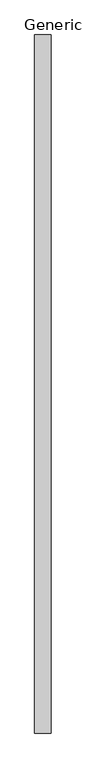
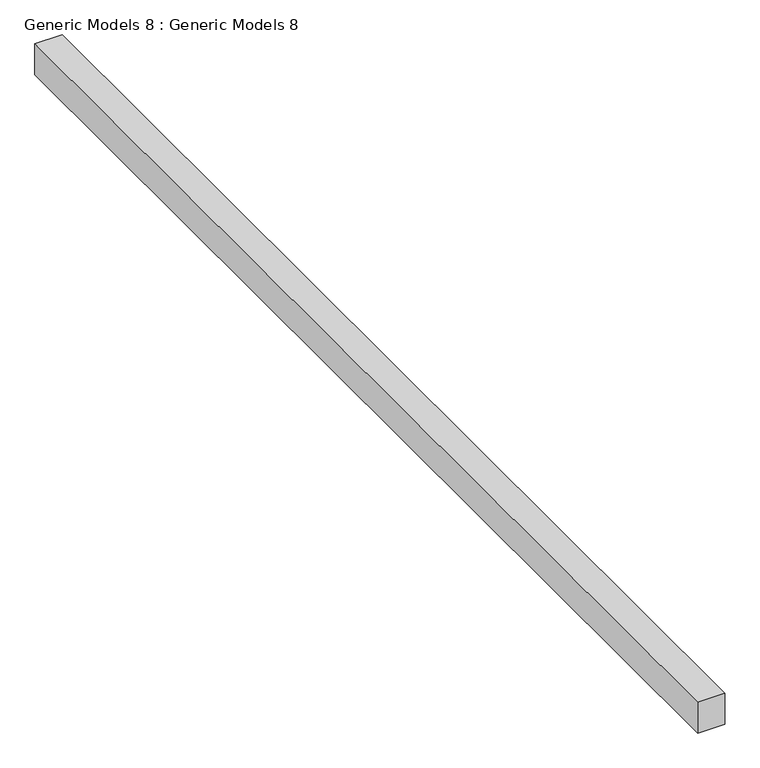
"""IFC4 building model written with IfcOpenShell, lengths in millimetres: proxy geometry, Generic Models 8 : Generic Models 8."""

from ifc_helpers import new_model, si_unit, frame, origin, place, context, project, spatial, polyline, outline, extrude, source, transform, mapped, element, save


def generic_models_8_generic_models_8_16792cbe(model_context):
    return source(origin(), model_context, "Body", "SweptSolid", [
        extrude(outline(polyline([(-14138.2638778, 4522.2475408), (-14138.2638778, 17411.9959632), (-13833.4638778, 17411.9959632), (-13833.4638778, 4522.2475408), (-14138.2638778, 4522.2475408)])), frame((0.0, 0.0, 18533.4806122), z_axis=(0.0, 0.0, 1.0), x_axis=(1.0, 0.0, 0.0)), (0.0, 0.0, 1.0), 364.1193878),
    ])


if __name__ == "__main__":
    model = new_model("IFC4")
    model_context = context("Model", 3, world=origin())
    ifc_project = project(units=[si_unit("LENGTHUNIT", "METRE", prefix="MILLI")], contexts=[model_context])
    site = spatial("IfcSite", under=ifc_project)
    building = spatial("IfcBuilding", under=site)
    placement = place(None, origin())
    generic_models_8_generic_models_8_shape = generic_models_8_generic_models_8_16792cbe(model_context)
    element("IfcBuildingElementProxy", 1, Name="Generic Models 8 : Generic Models 8", ObjectType="Generic Models 8 : Generic Models 8", at=placement, inside=building, context=model_context, shape_type="MappedRepresentation", body=[
        mapped(generic_models_8_generic_models_8_shape, transform((0.0, 0.0, 0.0), x_axis=(1.0, 0.0, 0.0), y_axis=(0.0, 1.0, 0.0), z_axis=(0.0, 0.0, 1.0))),
    ])
    save(model, "model.ifc")
